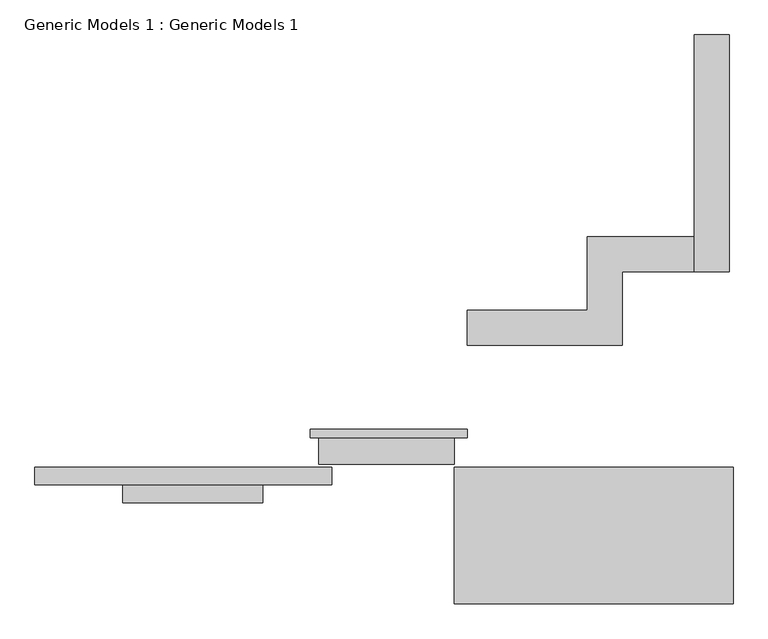
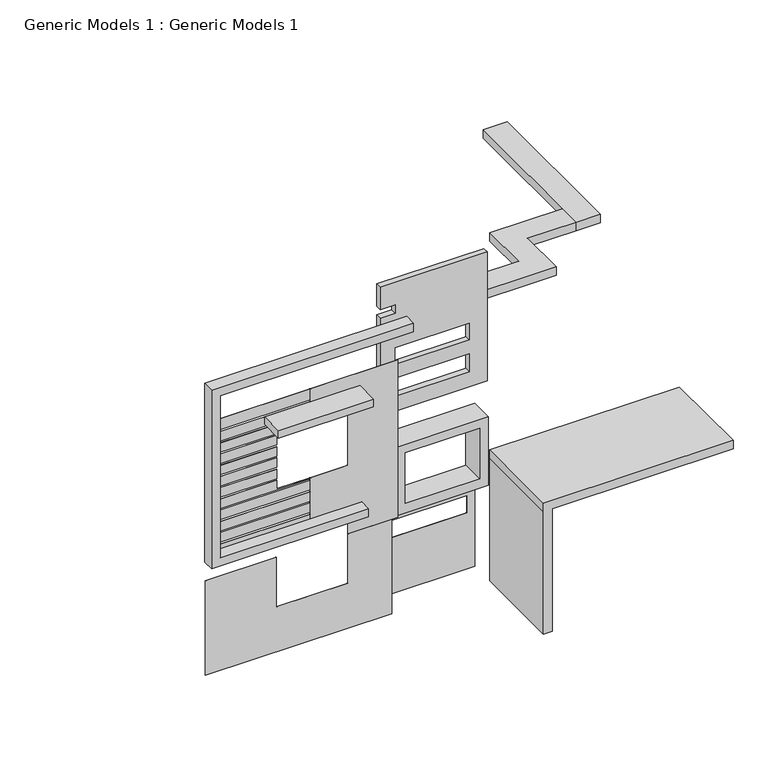
"""IFC4 building model written with IfcOpenShell, lengths in millimetres: proxy geometry, Generic Models 1 : Generic Models 1."""

from ifc_helpers import new_model, si_unit, frame, origin, place, context, project, spatial, polyline, outline, extrude, faceted_brep, source, transform, mapped, element, save


def generic_models_1_generic_models_1_ca1a1a43(model_context):
    return source(origin(), model_context, "Body", "SolidModel", [
        extrude(outline(polyline([(6832.6, -4858.2657257), (6273.8, -4858.2657257), (6273.8, -3894.7749552), (4419.6, -3894.7749552), (4419.6, -4858.2657257), (3302.0, -4858.2657257), (3302.0, -3539.1749552), (3073.4, -3539.1749552), (3073.4, -3894.7749552), (2558.0875781, -3894.7749552), (2558.0875781, -2608.6564961), (6832.6, -2608.6564961), (6832.6, -4858.2657257)])), frame((0.0, -726.4441274, 0.0), z_axis=(0.0, 1.0, 0.0), x_axis=(0.0, 0.0, 1.0)), (0.0, 0.0, 1.0), 5.0601562),
        extrude(outline(polyline([(-4858.2657257, -726.4441274), (-7336.4749552, -726.4441274), (-7336.4749552, -721.3839711), (-4858.2657257, -721.3839711), (-4858.2657257, -726.4441274)])), frame((0.0, 0.0, 6527.8), z_axis=(0.0, 0.0, 1.0), x_axis=(1.0, 0.0, 0.0)), (0.0, 0.0, 1.0), 304.8),
        extrude(outline(polyline([(-4858.2657257, -726.4441274), (-7336.4749552, -726.4441274), (-7336.4749552, -721.3839711), (-4858.2657257, -721.3839711), (-4858.2657257, -726.4441274)])), frame((0.0, 0.0, 3302.0), z_axis=(0.0, 0.0, 1.0), x_axis=(1.0, 0.0, 0.0)), (0.0, 0.0, 1.0), 127.0),
        extrude(outline(polyline([(4419.6, -4858.2657257), (4419.6, -5723.5749552), (4648.2, -5723.5749552), (4648.2, -7336.4749552), (4394.2, -7336.4749552), (4394.2, -4858.2657257), (4419.6, -4858.2657257)])), frame((0.0, -726.4441274, 0.0), z_axis=(0.0, 1.0, 0.0), x_axis=(0.0, 0.0, 1.0)), (0.0, 0.0, 1.0), 5.0601562),
        extrude(outline(polyline([(6273.8, -5723.5749552), (6273.8, -4858.2657257), (6477.0, -4858.2657257), (6477.0, -7336.4749552), (6223.0, -7336.4749552), (6223.0, -5723.5749552), (6273.8, -5723.5749552)])), frame((0.0, -726.4441274, 0.0), z_axis=(0.0, 1.0, 0.0), x_axis=(0.0, 0.0, 1.0)), (0.0, 0.0, 1.0), 5.0601562),
        extrude(outline(polyline([(-5723.5749552, -726.4441274), (-7336.4749552, -726.4441274), (-7336.4749552, -721.3839711), (-5723.5749552, -721.3839711), (-5723.5749552, -726.4441274)])), frame((0.0, 0.0, 5918.2), z_axis=(0.0, 0.0, 1.0), x_axis=(1.0, 0.0, 0.0)), (0.0, 0.0, 1.0), 254.0),
        extrude(outline(polyline([(-5723.5749552, -726.4441274), (-7336.4749552, -726.4441274), (-7336.4749552, -721.3839711), (-5723.5749552, -721.3839711), (-5723.5749552, -726.4441274)])), frame((0.0, 0.0, 5613.4), z_axis=(0.0, 0.0, 1.0), x_axis=(1.0, 0.0, 0.0)), (0.0, 0.0, 1.0), 254.0),
        extrude(outline(polyline([(-5723.5749552, -726.4441274), (-7336.4749552, -726.4441274), (-7336.4749552, -721.3839711), (-5723.5749552, -721.3839711), (-5723.5749552, -726.4441274)])), frame((0.0, 0.0, 5308.6), z_axis=(0.0, 0.0, 1.0), x_axis=(1.0, 0.0, 0.0)), (0.0, 0.0, 1.0), 254.0),
        extrude(outline(polyline([(-5723.5749552, -726.4441274), (-7336.4749552, -726.4441274), (-7336.4749552, -721.3839711), (-5723.5749552, -721.3839711), (-5723.5749552, -726.4441274)])), frame((0.0, 0.0, 5003.8), z_axis=(0.0, 0.0, 1.0), x_axis=(1.0, 0.0, 0.0)), (0.0, 0.0, 1.0), 254.0),
        extrude(outline(polyline([(-5723.5749552, -726.4441274), (-7336.4749552, -726.4441274), (-7336.4749552, -721.3839711), (-5723.5749552, -721.3839711), (-5723.5749552, -726.4441274)])), frame((0.0, 0.0, 4699.0), z_axis=(0.0, 0.0, 1.0), x_axis=(1.0, 0.0, 0.0)), (0.0, 0.0, 1.0), 254.0),
        extrude(outline(polyline([(-4858.2657257, -726.4441274), (-7336.4749552, -726.4441274), (-7336.4749552, -721.3839711), (-4858.2657257, -721.3839711), (-4858.2657257, -726.4441274)])), frame((0.0, 0.0, 4089.4), z_axis=(0.0, 0.0, 1.0), x_axis=(1.0, 0.0, 0.0)), (0.0, 0.0, 1.0), 254.0),
        extrude(outline(polyline([(-4858.2657257, -726.4441274), (-7336.4749552, -726.4441274), (-7336.4749552, -721.3839711), (-4858.2657257, -721.3839711), (-4858.2657257, -726.4441274)])), frame((0.0, 0.0, 3784.6), z_axis=(0.0, 0.0, 1.0), x_axis=(1.0, 0.0, 0.0)), (0.0, 0.0, 1.0), 254.0),
        extrude(outline(polyline([(-4858.2657257, -726.4441274), (-7336.4749552, -726.4441274), (-7336.4749552, -721.3839711), (-4858.2657257, -721.3839711), (-4858.2657257, -726.4441274)])), frame((0.0, 0.0, 3479.8), z_axis=(0.0, 0.0, 1.0), x_axis=(1.0, 0.0, 0.0)), (0.0, 0.0, 1.0), 254.0),
        faceted_brep([(-7565.0749552, -1026.1839711, 3073.4), (-3539.1749552, -1026.1839711, 3073.4), (-3539.1749552, -1026.1839711, 3302.0), (-7336.4749552, -1026.1839711, 3302.0), (-7336.4749552, -1026.1839711, 7696.2), (-2383.4749552, -1026.1839711, 7696.2), (-2383.4749552, -1026.1839711, 7924.8), (-7565.0749552, -1026.1839711, 7924.8), (-7565.0749552, -721.3839711, 3073.4), (-7565.0749552, -721.3839711, 7924.8), (-2383.4749552, -721.3839711, 7924.8), (-2383.4749552, -721.3839711, 7696.2), (-7336.4749552, -721.3839711, 7696.2), (-7336.4749552, -721.3839711, 6527.8), (-7336.4749552, -721.3839711, 6477.0), (-7336.4749552, -721.3839711, 6223.0), (-7336.4749552, -721.3839711, 6172.2), (-7336.4749552, -721.3839711, 5918.2), (-7336.4749552, -721.3839711, 5867.4), (-7336.4749552, -721.3839711, 5613.4), (-7336.4749552, -721.3839711, 5562.6), (-7336.4749552, -721.3839711, 5308.6), (-7336.4749552, -721.3839711, 5257.8), (-7336.4749552, -721.3839711, 5003.8), (-7336.4749552, -721.3839711, 4953.0), (-7336.4749552, -721.3839711, 4699.0), (-7336.4749552, -721.3839711, 4648.2), (-7336.4749552, -721.3839711, 4394.2), (-7336.4749552, -721.3839711, 4343.4), (-7336.4749552, -721.3839711, 4089.4), (-7336.4749552, -721.3839711, 4038.6), (-7336.4749552, -721.3839711, 3784.6), (-7336.4749552, -721.3839711, 3733.8), (-7336.4749552, -721.3839711, 3479.8), (-7336.4749552, -721.3839711, 3429.0), (-7336.4749552, -721.3839711, 3302.0), (-3539.1749552, -721.3839711, 3302.0), (-3539.1749552, -721.3839711, 3073.4)], [[[0, 1, 2, 3, 4, 5, 6, 7]], [[8, 9, 10, 11, 12, 13, 14, 15, 16, 17, 18, 19, 20, 21, 22, 23, 24, 25, 26, 27, 28, 29, 30, 31, 32, 33, 34, 35, 36, 37]], [[1, 0, 8, 37]], [[2, 1, 37, 36]], [[3, 2, 36, 35]], [[4, 3, 35, 34, 33, 32, 31, 30, 29, 28, 27, 26, 25, 24, 23, 22, 21, 20, 19, 18, 17, 16, 15, 14, 13, 12]], [[0, 7, 9, 8]], [[5, 4, 12, 11]], [[6, 5, 11, 10]], [[7, 6, 10, 9]]]),
        extrude(outline(polyline([(7696.2, -2764.4749552), (5039.9421734, -2764.4749552), (5039.9421734, -21.2749552), (8534.4, -21.2749552), (8534.4, -2764.4749552), (7924.8, -2764.4749552), (7924.8, -2383.4749552), (7696.2, -2383.4749552), (7696.2, -2764.4749552)]), holes=[polyline([(5927.3906231, -478.4749552), (5446.3786483, -478.4749552), (5446.3786483, -2380.0564961), (5927.3906231, -2380.0564961), (5927.3906231, -478.4749552)]), polyline([(6765.5847346, -478.4749552), (6307.1112081, -478.4749552), (6307.1112081, -2380.0564961), (6765.5847346, -2380.0564961), (6765.5847346, -478.4749552)])]), frame((0.0, -207.0339711, 0.0), z_axis=(0.0, 1.0, 0.0), x_axis=(0.0, 0.0, 1.0)), (0.0, 0.0, 1.0), 152.4),
        extrude(outline(polyline([(2558.0875781, -249.8749552), (4419.6, -249.8749552), (4419.6, -2608.6564961), (2558.0875781, -2608.6564961), (2558.0875781, -249.8749552)]), holes=[polyline([(4191.0, -478.4749552), (2819.4, -478.4749552), (2819.4, -2380.0564961), (4191.0, -2380.0564961), (4191.0, -478.4749552)])]), frame((0.0, -664.2339711, 0.0), z_axis=(0.0, 1.0, 0.0), x_axis=(0.0, 0.0, 1.0)), (0.0, 0.0, 1.0), 609.6),
        extrude(outline(polyline([(2558.0875781, -249.8749552), (2558.0875781, -2764.4749552), (0.0, -2764.4749552), (0.0, -249.8749552), (2558.0875781, -249.8749552)]), holes=[polyline([(1981.2, -459.4249552), (1524.0, -459.4249552), (1524.0, -2593.0249552), (1981.2, -2593.0249552), (1981.2, -459.4249552)])]), frame((0.0, -57.2136586, 0.0), z_axis=(0.0, 1.0, 0.0), x_axis=(0.0, 0.0, 1.0)), (0.0, 0.0, 1.0), 2.5796875),
        extrude(outline(polyline([(-3589.9749552, -1336.0441274), (-6028.3749552, -1336.0441274), (-6028.3749552, -726.4441274), (-3589.9749552, -726.4441274), (-3589.9749552, -1336.0441274)])), frame((0.0, 0.0, 6273.8), z_axis=(0.0, 0.0, 1.0), x_axis=(1.0, 0.0, 0.0)), (0.0, 0.0, 1.0), 203.2),
        extrude(outline(polyline([(4550.7250448, 6822.4160289), (4550.7250448, 2688.5660289), (3941.1250448, 2688.5660289), (3941.1250448, 6822.4160289), (4550.7250448, 6822.4160289)])), frame((0.0, 0.0, 5969.0), z_axis=(0.0, 0.0, 1.0), x_axis=(1.0, 0.0, 0.0)), (0.0, 0.0, 1.0), 228.6),
        extrude(outline(polyline([(-21.2749552, 1412.2160289), (-21.2749552, 2021.8160289), (2074.2250448, 2021.8160289), (2074.2250448, 3298.1660289), (3941.1250448, 3298.1660289), (3941.1250448, 2688.5660289), (2683.8250448, 2688.5660289), (2683.8250448, 1412.2160289), (-21.2749552, 1412.2160289)])), frame((0.0, 0.0, 5969.0), z_axis=(0.0, 0.0, 1.0), x_axis=(1.0, 0.0, 0.0)), (0.0, 0.0, 1.0), 228.6),
        extrude(outline(polyline([(0.0, -21.2749552), (3327.4, -21.2749552), (3327.4, 4616.3546353), (3556.0, 4616.3546353), (3556.0, -249.8749552), (3327.4, -249.8749552), (0.0, -249.8749552), (0.0, -21.2749552)])), frame((0.0, -3105.3092797, 0.0), z_axis=(0.0, 1.0, 0.0), x_axis=(0.0, 0.0, 1.0)), (0.0, 0.0, 1.0), 2383.9253085),
        extrude(outline(polyline([(0.0, -7549.1999552), (0.0, -2764.4749552), (2558.0875781, -2764.4749552), (2558.0875781, -3894.7749552), (1219.2, -3894.7749552), (1219.2, -5723.5749552), (2558.0875781, -5723.5749552), (2558.0875781, -7549.1999552), (0.0, -7549.1999552)])), frame((0.0, -723.9636586, 0.0), z_axis=(0.0, 1.0, 0.0), x_axis=(0.0, 0.0, 1.0)), (0.0, 0.0, 1.0), 2.5796875),
    ])


if __name__ == "__main__":
    model = new_model("IFC4")
    model_context = context("Model", 3, world=origin())
    ifc_project = project(units=[si_unit("LENGTHUNIT", "METRE", prefix="MILLI")], contexts=[model_context])
    site = spatial("IfcSite", under=ifc_project)
    building = spatial("IfcBuilding", under=site)
    placement = place(None, origin())
    generic_models_1_generic_models_1_shape = generic_models_1_generic_models_1_ca1a1a43(model_context)
    element("IfcBuildingElementProxy", 1, Name="Generic Models 1 : Generic Models 1", ObjectType="Generic Models 1 : Generic Models 1", at=placement, inside=building, context=model_context, shape_type="MappedRepresentation", body=[
        mapped(generic_models_1_generic_models_1_shape, transform((0.0, 0.0, 0.0), x_axis=(1.0, 0.0, 0.0), y_axis=(0.0, 1.0, 0.0), z_axis=(0.0, 0.0, 1.0))),
    ])
    save(model, "model.ifc")

# Revit data of these elements
# Element 1 (IfcBuildingElementProxy, "Generic Models 1 : Generic Models 1")
#   Materials on its faces: "Door - Frame", "Laminate, Linen, Matte", "Ash colour", "Linen, White"
# Materials
#   "Door - Frame": colour RGB 118 70 51, transparency 0, Cost = 0
#   "Laminate, Linen, Matte": class "Plastic", colour RGB 198 189 176, transparency 0, Description = "Plastic Laminate - Linen, Matte", Cost = 0
#   "Ash colour": class "Generic", colour RGB 94 94 94, transparency 0, Cost = 0
#   "Linen, White": class "Textile", colour RGB 206 206 206, transparency 0, Description = "Linen, white", Cost = 0
